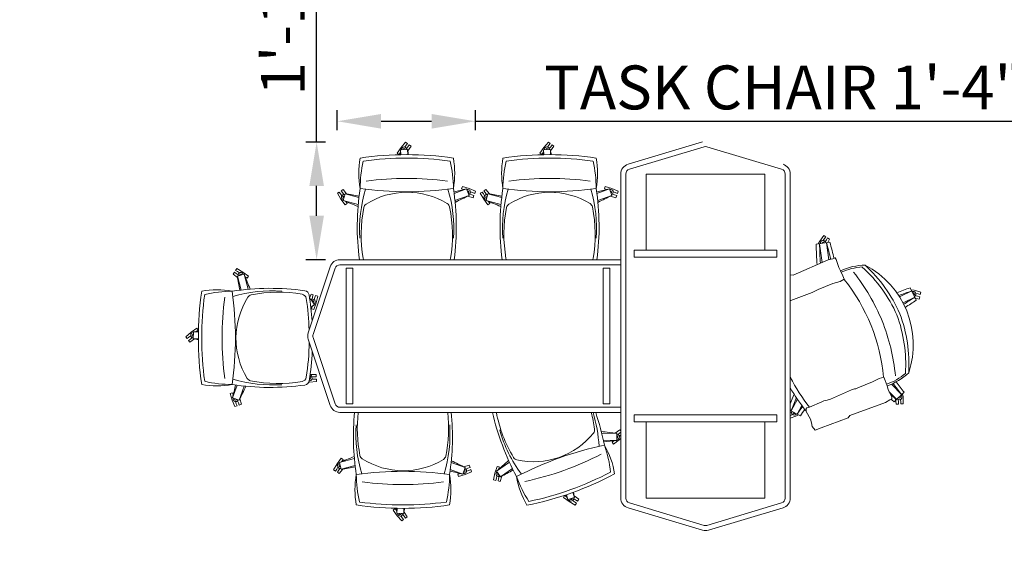
# Model space of a CAD drawing. Units: inches. Extents: x -100 to 766, y -562 to 63.
# Tile 5 of 11: x 268 to 380, y -383 to -323. Entities that reach past the tile are written whole.
import ezdxf

# ---------------------------------------------------------------- set-up
doc = ezdxf.new("R2010")
doc.units = ezdxf.units.IN
doc.layers.add('A-ANNO-DIMS', color=2, linetype='Continuous', lineweight=18)
doc.layers.add('furn', color=8, linetype='Continuous', lineweight=13)
doc.styles.get("Standard").update_dxf_attribs({"font": 'arial.ttf'})
doc.dimstyles.new('ISO-25', dxfattribs={"dimtxt": 5, "dimasz": 5, "dimexe": 1.25, "dimexo": 0.625, "dimtad": 1, "dimlunit": 3, "dimtxsty": 'Standard', "dimcen": 2.5, "dimadec": 0, "dimazin": 0, "dimtfac": 1, "dimtmove": 0, "dimatfit": 3, "dimfxl": 1, "dimfxlon": 1, "dimarcsym": 0})

# ---------------------------------------------------------------- blocks, each defined once
blk = doc.blocks.new('CHAIR-OFFICE')
for p, q in [((6.82, 12.16), (7.28, 12.81)), ((7.22, 12.53), (8.02, 12.56)), ((7.22, 12.53), (7.25, 11.97)), ((7.28, 12.81), (7.79, 13.42)), ((7.84, 13.05), (7.68, 12.84)), ((7.79, 13.42), (8, 13.25)), ((8, 13.25), (7.84, 13.05)), ((8.05, 12.88), (7.89, 12.68)), ((8.02, 12.56), (8.04, 11.98)), ((8.04, 12.4), (8.42, 12.93)), ((8.21, 13.09), (8.05, 12.88)), ((8.42, 12.93), (8.21, 13.09)), ((7.03, 12), (6.82, 12.16)), ((7.19, 12.21), (7.03, 12)), ((7.2, 12.22), (7.19, 12.21)), ((0.66, 8.02), (0.44, 7.87)), ((0.44, 7.87), (0.59, 7.65)), ((1.05, 7.5), (0.66, 8.02)), ((14.74, 8.08), (13.32, 7.55)), ((14.18, 8.1), (14.27, 8.35)), ((14.43, 8.01), (14.18, 8.1)), ((14.27, 8.35), (15.03, 8.12)), ((14.43, 8.01), (14.43, 8.01)), ((14.74, 8.08), (15.02, 7.34)), ((15.03, 8.12), (15.76, 7.81)), ((0, 7.57), (0.22, 7.72)), ((0.41, 6.89), (0, 7.57)), ((0.22, 7.72), (0.37, 7.5)), ((0.37, 7.5), (0.51, 7.29)), ((0.89, 6.26), (0.41, 6.89)), ((0.59, 7.65), (0.73, 7.44)), ((0.67, 6.76), (0.88, 7.52)), ((0.67, 6.76), (2.38, 6.28)), ((0.88, 7.52), (2.46, 7.08)), ((15.02, 7.34), (13.41, 6.74)), ((14.87, 7.26), (15.49, 7.07)), ((15.33, 7.4), (15.09, 7.49)), ((15.42, 7.65), (15.18, 7.74)), ((15.58, 7.32), (15.33, 7.4)), ((15.67, 7.56), (15.42, 7.65)), ((15.49, 7.07), (15.58, 7.32)), ((15.76, 7.81), (15.67, 7.56)), ((1.11, 6.41), (0.89, 6.26)), ((0.96, 6.64), (0.96, 6.63)), ((0.96, 6.63), (1.11, 6.41))]:
    blk.add_line(p, q)
for centre, radius, start, end in [((54.31, 8.3), 47.27, 174.8588, 175.5421), ((7.62, 12.55), 0.303, 2.3066, 182.3066), ((7.62, 12.55), 0.132, 2.3066, 182.3066), ((-38.57, 4.55), 47.27, 9.0337, 9.7544), ((25.26, -38.01), 47.27, 102.8588, 104.6675), ((14.88, 7.71), 0.303, 290.3066, 110.3066), ((0.77, 7.14), 0.303, 74.3066, 254.3066), ((0.77, 7.14), 0.132, 74.3066, 254.3066), ((19.24, 50.23), 47.27, 246.8588, 249.0775), ((-5.9, -39.26), 47.27, 79.7853, 81.7544), ((-7, 49.17), 47.27, 295.6055, 297.7544), ((14.88, 7.71), 0.132, 290.3066, 110.3066)]:
    blk.add_arc(centre, radius, start, end)
at = {"ltscale": 0.7}
for centre, radius, start, end in [((12.2, 9.85), 9.75, 169.7192, 190.2808), ((7.92, -24.77), 36.75, 81.6807, 98.3193), ((16.39, 8.11), 13.79, 166.8278, 180), ((7.92, -24.77), 36.36, 82.1689, 97.8311), ((-0.55, 8.11), 13.79, 0, 13.1722), ((3.64, 9.85), 9.75, 349.7192, 10.2808), ((7.92, -24.77), 34.04, 82.1689, 97.8311), ((30.98, 3.76), 28.71, 171.2841, 187.5243), ((18.22, 3.49), 15.68, 163.1781, 183.7805), ((7.92, 47.15), 39.4, 262.2438, 277.7562), ((-2.39, 3.49), 15.68, 356.2195, 16.8219), ((-15.14, 3.76), 28.71, 352.4757, 8.7159), ((7.96, -1.07), 8.76, 58.484, 122.3392), ((18.36, 2.85), 15.65, 168.5812, 189.9952), ((3.59, 5.84), 0.58, 122.3392, 168.5812), ((12.24, 5.9), 0.58, 11.6599, 58.484), ((-2.52, 2.85), 15.65, 350.0048, 11.6599), ((3.52, 0.24), 0.58, 189.9952, 204.0918), ((12.32, 0.24), 0.58, 335.9082, 350.0048)]:
    blk.add_arc(centre, radius, start, end, dxfattribs=at)
blk = doc.blocks.new('*D32')
at = {"layer": 'A-ANNO-DIMS', "color": 0, "lineweight": -2, "transparency": 16777216}
for p, q in [((304.17, -335.87), (304.17, -333.62)), ((319.93, -335.87), (319.93, -333.62)), ((309.17, -334.87), (314.93, -334.87)), ((319.93, -334.87), (400.64, -334.87))]:
    blk.add_line(p, q, dxfattribs=at)
at = {"layer": 'A-ANNO-DIMS', "color": 0, "transparency": 16777216}
for points in [[(309.17, -334.04), (309.17, -335.71), (304.17, -334.87)], [(314.93, -334.04), (314.93, -335.71), (319.93, -334.87)]]:
    blk.add_solid(points, dxfattribs=at)
at = {"layer": 'Defpoints', "color": 0, "transparency": 16777216}
for p in [(319.93, -334.87), (304.17, -337.24), (319.93, -337.24)]:
    blk.add_point(p, dxfattribs=at)
at = {"layer": 'A-ANNO-DIMS', "color": 0, "transparency": 16777216, "insert": (362.79, -331.66), "char_height": 5, "attachment_point": 5}
blk.add_mtext('TASK CHAIR 1\'-4" TYP.', dxfattribs=at)
blk = doc.blocks.new('*D33')
at = {"layer": 'A-ANNO-DIMS', "color": 0, "lineweight": -2, "transparency": 16777216}
for p, q in [((301.81, -337.24), (301.81, -289.33)), ((302.81, -337.24), (300.56, -337.24)), ((301.81, -345.65), (301.81, -342.24)), ((302.81, -350.65), (300.56, -350.65))]:
    blk.add_line(p, q, dxfattribs=at)
at = {"layer": 'A-ANNO-DIMS', "color": 0, "transparency": 16777216}
for points in [[(300.98, -342.24), (302.64, -342.24), (301.81, -337.24)], [(300.98, -345.65), (302.64, -345.65), (301.81, -350.65)]]:
    blk.add_solid(points, dxfattribs=at)
at = {"layer": 'Defpoints', "color": 0, "transparency": 16777216}
for p in [(301.81, -337.24), (304.17, -337.24), (304.17, -350.65)]:
    blk.add_point(p, dxfattribs=at)
at = {"layer": 'A-ANNO-DIMS', "color": 0, "transparency": 16777216, "insert": (298.6, -310.78), "char_height": 5, "attachment_point": 5, "rotation": 90}
blk.add_mtext('1\'-1 1/2" TYP.', dxfattribs=at)
blk = doc.blocks.new('*D49')
at = {"layer": 'A-ANNO-DIMS', "color": 0, "lineweight": -2, "transparency": 16777216}
for p, q in [((-88.51, -356.21), (-90.76, -356.21)), ((-89.51, -361.21), (-89.51, -417.21)), ((-88.51, -422.21), (-90.76, -422.21))]:
    blk.add_line(p, q, dxfattribs=at)
at = {"layer": 'A-ANNO-DIMS', "color": 0, "transparency": 16777216}
for points in [[(-90.35, -361.21), (-88.68, -361.21), (-89.51, -356.21)], [(-90.35, -417.21), (-88.68, -417.21), (-89.51, -422.21)]]:
    blk.add_solid(points, dxfattribs=at)
at = {"layer": 'Defpoints', "color": 0, "transparency": 16777216}
for p in [(562.39, -356.21), (-89.51, -422.21), (562.39, -422.21)]:
    blk.add_point(p, dxfattribs=at)
at = {"layer": 'A-ANNO-DIMS', "color": 0, "transparency": 16777216, "insert": (-92.69, -389.21), "char_height": 5, "attachment_point": 5, "rotation": 90}
blk.add_mtext('5\'-6"', dxfattribs=at)
blk = doc.blocks.new('*D51')
at = {"layer": 'A-ANNO-DIMS', "color": 0, "lineweight": -2, "transparency": 16777216}
for p, q in [((-88.51, -308.21), (-90.76, -308.21)), ((-89.51, -313.21), (-89.51, -339.21)), ((-88.51, -344.21), (-90.76, -344.21))]:
    blk.add_line(p, q, dxfattribs=at)
at = {"layer": 'A-ANNO-DIMS', "color": 0, "transparency": 16777216}
for points in [[(-90.35, -313.21), (-88.68, -313.21), (-89.51, -308.21)], [(-90.35, -339.21), (-88.68, -339.21), (-89.51, -344.21)]]:
    blk.add_solid(points, dxfattribs=at)
at = {"layer": 'Defpoints', "color": 0, "transparency": 16777216}
for p in [(598.6, -308.21), (-89.51, -344.21), (598.6, -344.21)]:
    blk.add_point(p, dxfattribs=at)
at = {"layer": 'A-ANNO-DIMS', "color": 0, "transparency": 16777216, "insert": (-92.69, -326.21), "char_height": 5, "attachment_point": 5, "rotation": 90}
blk.add_mtext('3\'-0"', dxfattribs=at)
blk = doc.blocks.new('*D70')
at = {"layer": 'A-ANNO-DIMS', "color": 0, "lineweight": -2, "transparency": 16777216}
for p, q in [((-88.51, -376.85), (-90.76, -376.85)), ((-89.51, -381.85), (-89.51, -419.34)), ((-88.51, -424.34), (-90.76, -424.34))]:
    blk.add_line(p, q, dxfattribs=at)
at = {"layer": 'A-ANNO-DIMS', "color": 0, "transparency": 16777216}
for points in [[(-90.35, -381.85), (-88.68, -381.85), (-89.51, -376.85)], [(-90.35, -419.34), (-88.68, -419.34), (-89.51, -424.34)]]:
    blk.add_solid(points, dxfattribs=at)
at = {"layer": 'Defpoints', "color": 0, "transparency": 16777216}
for p in [(679.5, -376.85), (-89.51, -424.34), (679.5, -424.34)]:
    blk.add_point(p, dxfattribs=at)
at = {"layer": 'A-ANNO-DIMS', "color": 0, "transparency": 16777216, "insert": (-92.73, -400.59), "char_height": 5, "attachment_point": 5, "rotation": 90}
blk.add_mtext('3\'-11 1/2"', dxfattribs=at)
blk = doc.blocks.new('*D73')
at = {"layer": 'A-ANNO-DIMS', "color": 0, "lineweight": -2, "transparency": 16777216}
for p, q in [((-88.51, -345.04), (-90.76, -345.04)), ((-89.51, -350.04), (-89.51, -401.82)), ((-88.51, -406.82), (-90.76, -406.82))]:
    blk.add_line(p, q, dxfattribs=at)
at = {"layer": 'A-ANNO-DIMS', "color": 0, "transparency": 16777216}
for points in [[(-90.35, -350.04), (-88.68, -350.04), (-89.51, -345.04)], [(-90.35, -401.82), (-88.68, -401.82), (-89.51, -406.82)]]:
    blk.add_solid(points, dxfattribs=at)
at = {"layer": 'Defpoints', "color": 0, "transparency": 16777216}
for p in [(475.3, -345.04), (-89.51, -406.82), (475.3, -406.82)]:
    blk.add_point(p, dxfattribs=at)
at = {"layer": 'A-ANNO-DIMS', "color": 0, "transparency": 16777216, "insert": (-92.69, -375.93), "char_height": 5, "attachment_point": 5, "rotation": 90}
blk.add_mtext('5\'-2"', dxfattribs=at)
blk = doc.blocks.new('*D80')
at = {"layer": 'A-ANNO-DIMS', "color": 0, "lineweight": -2, "transparency": 16777216}
for p, q in [((241.52, -558.16), (236.52, -558.16)), ((246.52, -557.16), (246.52, -559.41)), ((246.52, -558.16), (250.39, -558.16)), ((250.39, -557.16), (250.39, -559.41)), ((255.39, -558.16), (274.93, -558.16))]:
    blk.add_line(p, q, dxfattribs=at)
at = {"layer": 'A-ANNO-DIMS', "color": 0, "transparency": 16777216}
for points in [[(241.52, -557.32), (241.52, -558.99), (246.52, -558.16)], [(255.39, -557.32), (255.39, -558.99), (250.39, -558.16)]]:
    blk.add_solid(points, dxfattribs=at)
at = {"layer": 'Defpoints', "color": 0, "transparency": 16777216}
for p in [(246.52, -368.21), (250.39, -368.21), (250.39, -558.16)]:
    blk.add_point(p, dxfattribs=at)
at = {"layer": 'A-ANNO-DIMS', "color": 0, "transparency": 16777216, "insert": (267.66, -554.98), "char_height": 5, "attachment_point": 5}
blk.add_mtext('0\'-4"', dxfattribs=at)
blk = doc.blocks.new('*D87')
at = {"layer": 'A-ANNO-DIMS', "color": 0, "lineweight": -2, "transparency": 16777216}
for p, q in [((310.41, -557.16), (310.41, -559.41)), ((315.41, -558.16), (352.79, -558.16)), ((357.79, -557.16), (357.79, -559.41))]:
    blk.add_line(p, q, dxfattribs=at)
at = {"layer": 'A-ANNO-DIMS', "color": 0, "transparency": 16777216}
for points in [[(315.41, -557.32), (315.41, -558.99), (310.41, -558.16)], [(352.79, -557.32), (352.79, -558.99), (357.79, -558.16)]]:
    blk.add_solid(points, dxfattribs=at)
at = {"layer": 'Defpoints', "color": 0, "transparency": 16777216}
for p in [(310.41, -121.91), (357.79, -121.91), (357.79, -558.16)]:
    blk.add_point(p, dxfattribs=at)
at = {"layer": 'A-ANNO-DIMS', "color": 0, "transparency": 16777216, "insert": (334.1, -554.94), "char_height": 5, "attachment_point": 5}
blk.add_mtext('3\'-11 1/2"', dxfattribs=at)

msp = doc.modelspace()

# ---------------------------------------------------------------- linework, layer by layer
at = {"layer": 'furn', "ltscale": 0.2}
for p, q in [((337.331, -339.771), (345.839, -337.219)), ((337.498, -340.326), (346.006, -337.774)), ((346.339, -337.774), (354.847, -340.326)), ((336.504, -377.828), (336.504, -340.882)), ((337.084, -377.828), (337.084, -340.882)), ((355.26, -340.882), (355.26, -377.828)), ((355.84, -340.882), (355.84, -377.828)), ((300.855, -358.988), (303.369, -351.447)), ((304.469, -350.654), (336.504, -350.654)), ((304.469, -351.234), (336.504, -351.234)), ((336.504, -350.654), (336.504, -368.056)), ((301.405, -359.171), (303.919, -351.63)), ((303.369, -367.263), (300.855, -359.722)), ((303.919, -367.079), (301.405, -359.538)), ((336.504, -367.476), (304.469, -367.476)), ((336.504, -368.056), (304.469, -368.056)), ((346.006, -380.935), (337.498, -378.383)), ((354.847, -378.383), (346.339, -380.935)), ((345.839, -381.491), (337.331, -378.939)), ((355.013, -378.939), (346.506, -381.491))]:
    msp.add_line(p, q, dxfattribs=at)
at = {"layer": 'furn', "ltscale": 0.4}
for p, q in [((339.405, -349.583), (339.405, -340.882)), ((339.405, -340.882), (349.073, -340.882)), ((349.073, -340.882), (352.94, -340.882)), ((352.94, -340.882), (352.94, -349.583)), ((338.051, -349.583), (354.293, -349.583)), ((338.051, -350.357), (338.051, -349.583)), ((354.293, -350.357), (338.051, -350.357)), ((352.94, -349.583), (339.405, -349.583)), ((354.293, -349.583), (354.293, -350.357)), ((305.944, -351.62), (305.171, -351.62)), ((305.171, -351.62), (305.171, -367.089)), ((305.944, -367.089), (305.944, -351.62)), ((335.259, -351.62), (334.486, -351.62)), ((334.486, -351.62), (334.486, -367.089)), ((335.259, -367.089), (335.259, -351.62)), ((305.171, -367.089), (305.944, -367.089)), ((334.486, -367.089), (335.259, -367.089)), ((354.293, -368.353), (338.051, -368.353)), ((338.051, -368.353), (338.051, -369.126)), ((354.293, -369.126), (354.293, -368.353)), ((338.051, -369.126), (354.293, -369.126)), ((339.405, -369.126), (339.405, -377.828)), ((352.94, -369.126), (339.405, -369.126)), ((352.94, -377.828), (352.94, -369.126)), ((339.405, -377.828), (349.073, -377.828)), ((349.073, -377.828), (352.94, -377.828))]:
    msp.add_line(p, q, dxfattribs=at)
at = {"layer": 'furn'}
for p, q in [((359.208, -348.542), (359.659, -347.889)), ((359.659, -347.889), (359.883, -348.028)), ((359.883, -348.028), (359.744, -348.253)), ((360.107, -348.167), (359.968, -348.392)), ((360.332, -348.306), (360.107, -348.167)), ((358.801, -348.885), (360.356, -348.657)), ((359.038, -348.85), (359.208, -348.542)), ((359.187, -348.829), (359.5, -350.966)), ((359.193, -349.143), (359.188, -349.15)), ((359.744, -348.253), (359.61, -348.469)), ((359.968, -348.392), (359.834, -348.608)), ((359.97, -348.714), (360.256, -350.66)), ((360.119, -348.692), (360.332, -348.306)), ((292.275, -352.3), (292.424, -352.082)), ((292.796, -352.694), (292.275, -352.3)), ((292.424, -352.082), (292.642, -352.23)), ((292.72, -351.645), (292.572, -351.864)), ((292.572, -351.864), (292.79, -352.012)), ((292.642, -352.23), (292.853, -352.374)), ((293.397, -352.058), (292.72, -351.645)), ((293.534, -352.311), (292.772, -352.525)), ((292.772, -352.525), (293.216, -354.107)), ((292.79, -352.012), (293.001, -352.155)), ((294.03, -352.535), (293.397, -352.058)), ((293.534, -352.311), (294.016, -354.025)), ((293.657, -352.601), (293.664, -352.605)), ((293.664, -352.605), (293.882, -352.754)), ((293.882, -352.754), (294.03, -352.535)), ((301.015, -355.043), (301.176, -354.575)), ((301.176, -354.575), (301.43, -354.649)), ((301.356, -354.902), (301.285, -355.147)), ((301.43, -354.649), (301.356, -354.902)), ((301.683, -354.722), (301.61, -354.976)), ((301.937, -354.796), (301.683, -354.722)), ((301.754, -355.567), (301.937, -354.796)), ((369.696, -354.207), (368.312, -354.893)), ((370.048, -354.917), (368.707, -355.581)), ((369.399, -354.31), (369.391, -354.308)), ((369.523, -353.858), (370.221, -355.266)), ((369.629, -354.072), (369.976, -354.139)), ((369.976, -354.139), (370.735, -354.366)), ((370.353, -354.816), (370.106, -354.755)), ((370.416, -354.559), (370.169, -354.499)), ((370.61, -354.878), (370.353, -354.816)), ((370.672, -354.622), (370.416, -354.559)), ((370.547, -355.135), (370.61, -354.878)), ((370.735, -354.366), (370.672, -354.622)), ((301.116, -355.116), (301.034, -355.171)), ((301.555, -355.775), (301.116, -355.116)), ((301.555, -355.775), (301.15, -356.046)), ((301.315, -355.99), (301.242, -356.243)), ((301.317, -355.982), (301.315, -355.99)), ((301.495, -356.317), (301.754, -355.567)), ((301.61, -354.976), (301.539, -355.22)), ((369.906, -355.011), (370.547, -355.135)), ((301.242, -356.243), (301.495, -356.317)), ((287.478, -358.921), (286.876, -359.437)), ((286.876, -359.437), (287.038, -359.646)), ((287.246, -359.484), (287.448, -359.328)), ((288.127, -358.466), (287.478, -358.921)), ((287.76, -358.869), (287.728, -359.66)), ((287.76, -358.869), (288.321, -358.892)), ((288.074, -358.842), (288.081, -358.837)), ((288.081, -358.837), (288.289, -358.675)), ((288.289, -358.675), (288.127, -358.466)), ((287.038, -359.646), (287.246, -359.484)), ((287.2, -359.854), (287.408, -359.692)), ((287.361, -360.063), (287.2, -359.854)), ((287.896, -359.689), (287.361, -360.063)), ((287.408, -359.692), (287.609, -359.536)), ((287.728, -359.66), (288.315, -359.684)), ((301.007, -364.136), (301.23, -363.853)), ((301.007, -364.136), (301.23, -363.853)), ((301.23, -363.853), (301.067, -363.725)), ((301.23, -363.853), (301.067, -363.725)), ((301.111, -363.731), (301.763, -363.743)), ((301.111, -363.731), (301.763, -363.743)), ((301.763, -363.743), (301.772, -364.007)), ((301.763, -363.743), (301.772, -364.007)), ((292.213, -366.387), (292.741, -364.961)), ((300.915, -364.598), (300.998, -364.599)), ((300.915, -364.598), (300.998, -364.599)), ((300.998, -364.599), (301.788, -364.535)), ((300.998, -364.599), (301.788, -364.535)), ((301.508, -364.015), (301.253, -364.023)), ((301.508, -364.015), (301.253, -364.023)), ((301.516, -364.279), (301.262, -364.287)), ((301.516, -364.279), (301.262, -364.287)), ((301.772, -364.007), (301.508, -364.015)), ((301.772, -364.007), (301.508, -364.015)), ((301.78, -364.271), (301.516, -364.279)), ((301.78, -364.271), (301.516, -364.279)), ((301.788, -364.535), (301.78, -364.271)), ((301.788, -364.535), (301.78, -364.271)), ((368.554, -366.044), (367.379, -364.841)), ((292.192, -365.824), (291.944, -365.913)), ((291.944, -365.913), (292.175, -366.671)), ((292.282, -366.072), (292.192, -365.824)), ((292.284, -366.08), (292.282, -366.072)), ((292.956, -366.661), (293.55, -365.057)), ((367.988, -366.597), (367.141, -365.731)), ((368.833, -365.771), (367.709, -366.87)), ((368.364, -365.792), (368.363, -365.784)), ((368.661, -365.938), (368.705, -366.288)), ((292.175, -366.671), (292.48, -367.403)), ((292.213, -366.387), (292.956, -366.661)), ((292.639, -367.065), (292.553, -366.826)), ((292.729, -367.314), (292.639, -367.065)), ((292.888, -366.976), (292.801, -366.736)), ((292.977, -367.224), (292.888, -366.976)), ((293.225, -367.135), (292.977, -367.224)), ((293.035, -366.51), (293.225, -367.135)), ((355.945, -367.894), (356.653, -366.543)), ((356.646, -368.262), (357.166, -367.27)), ((367.854, -366.491), (367.934, -367.139)), ((367.934, -367.139), (368.198, -367.12)), ((368.178, -366.857), (368.159, -366.602)), ((368.198, -367.12), (368.178, -366.857)), ((368.441, -366.837), (368.423, -366.583)), ((368.461, -367.1), (368.441, -366.837)), ((368.724, -367.081), (368.461, -367.1)), ((368.705, -366.288), (368.724, -367.081)), ((292.48, -367.403), (292.729, -367.314)), ((356.004, -367.734), (355.84, -367.811)), ((356.992, -368.443), (355.84, -367.84)), ((355.84, -368.122), (355.993, -368.059)), ((355.84, -368.407), (355.857, -368.4)), ((355.857, -368.4), (356.093, -368.304)), ((356.779, -368.332), (356.46, -368.481)), ((356.826, -368.004), (356.834, -368)), ((356.46, -368.481), (355.84, -368.699)), ((336.048, -370.46), (334.337, -370.442)), ((335.879, -370.437), (336.403, -370.047)), ((336.04, -371.252), (336.048, -370.46)), ((336.367, -370.418), (336.17, -370.58)), ((336.504, -370.647), (336.338, -370.784)), ((336.504, -370.305), (336.367, -370.418)), ((336.403, -370.047), (336.504, -370.17)), ((336.04, -371.252), (334.519, -371.236)), ((335.72, -371.294), (335.517, -371.462)), ((335.517, -371.462), (335.685, -371.665)), ((335.685, -371.665), (336.321, -371.192)), ((335.727, -371.288), (335.72, -371.294)), ((336.321, -371.192), (336.504, -371.024)), ((304.149, -373.918), (303.737, -374.595)), ((304.627, -373.285), (304.149, -373.918)), ((304.402, -373.781), (306.116, -373.3)), ((304.402, -373.781), (304.616, -374.543)), ((304.845, -373.433), (304.627, -373.285)), ((304.692, -373.658), (304.697, -373.651)), ((304.697, -373.651), (304.845, -373.433)), ((318.753, -374.359), (317.148, -373.765)), ((322.343, -374.756), (323.794, -373.725)), ((303.737, -374.595), (303.955, -374.743)), ((303.955, -374.743), (304.104, -374.525)), ((304.104, -374.525), (304.247, -374.314)), ((304.174, -374.891), (304.322, -374.673)), ((304.392, -375.04), (304.174, -374.891)), ((304.322, -374.673), (304.465, -374.462)), ((304.785, -374.519), (304.392, -375.04)), ((304.616, -374.543), (306.198, -374.099)), ((318.478, -375.102), (317.052, -374.574)), ((318.164, -375.033), (317.915, -375.123)), ((317.915, -375.123), (318.005, -375.371)), ((318.005, -375.371), (318.763, -375.14)), ((318.171, -375.031), (318.164, -375.033)), ((318.478, -375.102), (318.753, -374.359)), ((318.602, -374.28), (319.226, -374.09)), ((318.763, -375.14), (319.495, -374.835)), ((319.067, -374.427), (318.828, -374.514)), ((319.157, -374.676), (318.917, -374.762)), ((319.316, -374.338), (319.067, -374.427)), ((319.405, -374.586), (319.157, -374.676)), ((319.226, -374.09), (319.316, -374.338)), ((319.495, -374.835), (319.405, -374.586)), ((322.151, -374.97), (321.991, -375.747)), ((322.387, -374.213), (322.151, -374.97)), ((322.343, -374.756), (322.802, -375.402)), ((322.643, -374.279), (322.387, -374.213)), ((322.575, -374.543), (322.577, -374.535)), ((322.577, -374.535), (322.643, -374.279)), ((322.802, -375.402), (324.141, -374.45)), ((321.991, -375.747), (322.247, -375.813)), ((322.247, -375.813), (322.313, -375.557)), ((322.313, -375.557), (322.377, -375.311)), ((322.502, -375.879), (322.568, -375.623)), ((322.758, -375.945), (322.502, -375.879)), ((322.568, -375.623), (322.632, -375.377)), ((322.952, -375.322), (322.758, -375.945)), ((331.22, -377.743), (331.045, -377.183)), ((330.103, -377.547), (329.962, -377.77)), ((329.962, -377.77), (330.609, -378.228)), ((330.326, -377.689), (330.103, -377.547)), ((330.465, -377.98), (330.297, -377.444)), ((330.333, -377.694), (330.326, -377.689)), ((330.465, -377.98), (331.22, -377.743)), ((330.609, -378.228), (331.298, -378.62)), ((331.217, -378.256), (331.002, -378.119)), ((331.358, -378.033), (331.144, -377.897)), ((331.19, -377.575), (331.723, -377.952)), ((331.439, -378.398), (331.217, -378.256)), ((331.298, -378.62), (331.439, -378.398)), ((331.581, -378.175), (331.358, -378.033)), ((331.723, -377.952), (331.581, -378.175)), ((310.766, -379.026), (310.558, -379.188)), ((310.558, -379.188), (311.012, -379.838)), ((310.928, -379.235), (310.766, -379.026)), ((310.933, -379.241), (310.928, -379.235)), ((310.96, -379.555), (310.983, -378.994)), ((310.96, -379.555), (311.752, -379.587)), ((311.752, -379.587), (311.775, -379)), ((311.78, -379.419), (312.154, -379.954)), ((311.012, -379.838), (311.529, -380.439)), ((311.575, -380.069), (311.419, -379.867)), ((311.529, -380.439), (311.737, -380.277)), ((311.737, -380.277), (311.575, -380.069)), ((311.784, -379.907), (311.628, -379.706)), ((311.946, -380.115), (311.784, -379.907)), ((312.154, -379.954), (311.946, -380.115))]:
    msp.add_line(p, q, dxfattribs=at)
at = {"layer": 'furn', "ltscale": 0.7}
for p, q in [((356.171, -352.424), (360.148, -350.682)), ((360.148, -350.682), (360.701, -350.565)), ((360.701, -350.565), (360.95, -350.453)), ((360.95, -350.453), (361.085, -350.61)), ((361.085, -350.61), (361.382, -351.551)), ((361.382, -351.551), (361.584, -351.905)), ((355.84, -352.391), (355.882, -352.373)), ((355.882, -352.373), (356.171, -352.424)), ((361.584, -351.905), (361.836, -352.499)), ((361.836, -352.499), (361.988, -352.874)), ((360.708, -353.379), (359.006, -354.067)), ((361.522, -353.121), (360.708, -353.379)), ((361.988, -352.874), (361.522, -353.121)), ((358.358, -354.388), (355.891, -355.305)), ((358.654, -354.245), (358.358, -354.388)), ((358.804, -354.149), (358.654, -354.245)), ((359.006, -354.067), (358.804, -354.149)), ((355.891, -355.305), (355.84, -355.333)), ((365.237, -364.586), (363.535, -365.273)), ((366.002, -364.206), (365.237, -364.586)), ((366.508, -364.06), (366.002, -364.206)), ((366.66, -364.435), (366.508, -364.06)), ((366.891, -365.037), (366.66, -364.435)), ((366.992, -365.432), (366.891, -365.037)), ((362.846, -365.493), (360.435, -366.547)), ((363.158, -365.39), (362.846, -365.493)), ((363.333, -365.355), (363.158, -365.39)), ((363.535, -365.273), (363.333, -365.355)), ((367.432, -366.315), (366.992, -365.432)), ((359.451, -366.852), (358.054, -367.48)), ((359.681, -366.736), (359.451, -366.852)), ((360.062, -366.652), (359.681, -366.736)), ((360.435, -366.547), (360.062, -366.652)), ((362.638, -368.425), (366.708, -366.914)), ((366.708, -366.914), (367.187, -366.614)), ((367.187, -366.614), (367.445, -366.522)), ((367.445, -366.522), (367.432, -366.315)), ((357.739, -367.54), (357.642, -367.602)), ((357.642, -367.602), (357.655, -367.957)), ((357.655, -367.957), (358.134, -368.837)), ((357.894, -367.505), (357.739, -367.54)), ((358.054, -367.48), (357.894, -367.505)), ((358.134, -368.837), (358.276, -369.231)), ((358.276, -369.231), (358.35, -369.677)), ((359.368, -369.824), (362.465, -368.662)), ((362.465, -368.662), (362.638, -368.425)), ((358.35, -369.677), (358.685, -370.1)), ((358.685, -370.1), (359.368, -369.824))]:
    msp.add_line(p, q, dxfattribs=at)
at = {"layer": 'furn', "ltscale": 0.2}
for centre, radius, start, end in [((346.172, -338.33), 0.58, 73.30076, 106.69924), ((337.664, -340.882), 1.16, 106.69924, 180), ((337.664, -340.882), 0.58, 106.69924, 180), ((354.68, -340.882), 0.58, 0, 73.30076), ((354.68, -340.882), 1.16, 0, 73.30076), ((304.469, -351.814), 1.16, 90, 161.56505), ((304.469, -351.814), 0.58, 90, 161.56505), ((301.956, -359.355), 1.16, 161.56505, 198.43495), ((301.956, -359.355), 0.58, 161.56505, 198.43495), ((304.469, -366.896), 1.16, 198.43495, 270), ((304.469, -366.896), 0.58, 198.43495, 270), ((337.664, -377.828), 1.16, 180, 253.30076), ((337.664, -377.828), 0.58, 180, 253.30076), ((354.68, -377.828), 0.58, 286.69924, 0), ((354.68, -377.828), 1.16, 286.69924, 0), ((346.172, -380.38), 1.16, 253.30076, 286.69924), ((346.172, -380.38), 0.58, 253.30076, 286.69924)]:
    msp.add_arc(centre, radius, start, end, dxfattribs=at)
at = {"layer": 'furn'}
for centre, radius, start, end in [((406.454, -348.084), 47.66, 180.963, 183.7842), ((406.454, -348.084), 47.273, 180.90223, 183.61481), ((359.578, -348.771), 0.303, 8.35, 188.35), ((359.578, -348.771), 0.132, 8.35, 188.35), ((314.482, -361.583), 47.273, 13.41608, 15.79778), ((314.482, -361.583), 47.66, 13.41608, 15.73701), ((339.556, -345.745), 47.273, 188.2456, 190.21466), ((293.153, -352.418), 0.303, 15.69338, 195.69338), ((293.153, -352.418), 0.132, 15.69338, 195.69338), ((250.064, -370.889), 47.273, 20.92253, 23.14116), ((385.011, -398.931), 47.66, 108.963, 110.92121), ((385.011, -398.931), 47.273, 108.90223, 110.81068), ((343.751, -315.632), 47.273, 301.97499, 303.79778), ((369.872, -354.562), 0.303, 296.35, 116.35), ((369.872, -354.562), 0.132, 296.35, 116.35), ((322.021, -397.516), 47.273, 116.2456, 116.35919), ((270.453, -320.174), 47.273, 310.5051, 311.14116), ((301.336, -355.446), 0.303, 303.69338, 123.69338), ((301.336, -355.446), 0.132, 303.69338, 123.69338), ((343.751, -315.632), 47.66, 301.92298, 303.73701), ((287.744, -359.265), 0.303, 87.69338, 267.69338), ((287.744, -359.265), 0.132, 87.69338, 267.69338), ((291.996, -405.952), 47.273, 94.45788, 95.14116), ((295.738, -313.07), 47.273, 260.2456, 260.96632), ((300.984, -364.164), 0.303, 264.2846, 51.69338), ((300.984, -364.164), 0.303, 264.2846, 51.69338), ((267.365, -396.837), 47.273, 44.2456, 44.51988), ((267.365, -396.837), 47.273, 44.2456, 44.51988), ((338.301, -376.907), 47.273, 165.33246, 167.14116), ((300.984, -364.164), 0.132, 268.83313, 51.69338), ((300.984, -364.164), 0.132, 268.83313, 51.69338), ((330.751, -394.429), 47.273, 36.90223, 38.87325), ((330.751, -394.429), 47.66, 36.963, 38.7754), ((251.121, -344.647), 47.273, 332.2456, 334.39454), ((400.31, -384.219), 47.66, 157.49042, 158.91682), ((397.223, -329.448), 47.273, 230.72258, 231.79778), ((368.271, -366.32), 0.303, 224.35, 44.35), ((292.585, -366.524), 0.303, 159.69338, 339.69338), ((292.585, -366.524), 0.132, 159.69338, 339.69338), ((400.31, -384.219), 47.273, 157.81448, 159.79778), ((397.223, -329.448), 47.66, 231.14855, 231.73701), ((368.271, -366.32), 0.132, 224.35, 44.35), ((356.295, -368.078), 0.303, 152.35, 332.35), ((356.295, -368.078), 0.132, 152.35, 332.35), ((317.969, -341.081), 47.273, 324.90223, 326.19386), ((317.969, -341.081), 47.66, 324.963, 326.03412), ((329.435, -417.268), 47.273, 81.95831, 84.10725), ((336.044, -370.856), 0.303, 269.40608, 89.40608), ((330.398, -324.316), 47.273, 275.04516, 276.85386), ((336.044, -370.856), 0.132, 269.40608, 89.40608), ((304.509, -374.162), 0.303, 105.69338, 285.69338), ((304.509, -374.162), 0.132, 105.69338, 285.69338), ((322.981, -417.251), 47.273, 110.92253, 113.14116), ((296.739, -416.194), 47.273, 62.2456, 64.39454), ((354.495, -409.412), 47.273, 130.63523, 132.85386), ((297.837, -327.759), 47.273, 278.2456, 280.21466), ((328.999, -329.014), 47.273, 255.33246, 257.14116), ((318.615, -374.73), 0.303, 249.69338, 69.69338), ((318.615, -374.73), 0.132, 249.69338, 69.69338), ((322.573, -375.079), 0.303, 125.40608, 305.40608), ((322.573, -375.079), 0.132, 125.40608, 305.40608), ((300.639, -333.646), 47.273, 297.95831, 299.92736), ((284.659, -385.918), 47.273, 9.95831, 10.67903), ((373.359, -358.11), 47.273, 204.17059, 204.85386), ((330.842, -377.861), 0.303, 197.40608, 17.40608), ((330.842, -377.861), 0.132, 197.40608, 17.40608), ((358.043, -375.319), 47.273, 184.45788, 185.14116), ((311.356, -379.571), 0.303, 177.69338, 357.69338), ((311.356, -379.571), 0.132, 177.69338, 357.69338), ((265.162, -371.577), 47.273, 350.2456, 350.96632)]:
    msp.add_arc(centre, radius, start, end, dxfattribs=at)
at = {"layer": 'furn', "ltscale": 0.7}
for centre, radius, start, end in [((364.576, -358.552), 7.289, 91.40115, 114.23532), ((364.576, -358.552), 7.095, 94.08643, 114.23532), ((353.29, -363.438), 16.08, 23.80386, 48.00597), ((353.218, -363.476), 16.532, 23.78704, 47.55372), ((359.631, -360.333), 10.244, 341.74338, 62.26911), ((345.577, -366.013), 22.363, 22.00624, 38.583), ((345.577, -366.013), 21.01, 5.42949, 38.583), ((325.065, -359.563), 36.75, 171.68072, 188.31928), ((290.442, -363.84), 9.751, 79.71923, 100.28077), ((325.065, -359.563), 36.364, 172.16886, 187.83114), ((292.182, -368.031), 13.785, 90, 103.17216), ((325.065, -359.563), 34.043, 172.16886, 187.83114), ((296.532, -382.624), 28.71, 82.13296, 98.71594), ((253.142, -359.563), 39.4, 352.24381, 7.75619), ((296.797, -369.867), 15.676, 86.21948, 106.82194), ((301.365, -359.607), 8.759, 147.66079, 211.516), ((294.455, -355.232), 0.58, 101.41884, 147.66079), ((297.439, -370.006), 15.653, 80.00482, 101.41884), ((300.055, -355.162), 0.58, 8.67601, 80.00482), ((300.383, -354.759), 0.58, 9.35255, 82.13296), ((271.214, -359.563), 30.142, 3.6091, 9.35255), ((271.214, -359.563), 29.755, 1.69041, 8.67601), ((352.933, -362.561), 16.08, 356.2257, 20.42781), ((352.855, -362.584), 16.532, 356.67795, 20.44463), ((345.577, -366.013), 22.363, 5.42949, 22.00624), ((271.214, -359.563), 29.755, 351.32399, 359.06079), ((271.214, -359.563), 30.142, 350.64745, 357.06846), ((364.425, -358.178), 7.095, 289.77717, 309.92606), ((364.425, -358.178), 7.289, 289.77717, 312.61134), ((290.442, -355.286), 9.751, 259.71923, 280.28077), ((292.182, -351.095), 13.785, 256.82784, 270), ((296.532, -336.502), 28.71, 261.28406, 277.86704), ((296.797, -349.259), 15.676, 253.17806, 273.78052), ((294.393, -363.882), 0.58, 211.516, 258.34006), ((297.439, -349.12), 15.653, 258.34006, 279.99518), ((300.055, -363.964), 0.58, 279.99518, 351.32399), ((300.383, -364.367), 0.58, 277.86704, 350.64745), ((375.031, -354.131), 21.597, 207.30205, 218.17743), ((375.031, -354.131), 22.177, 210.07641, 218.17743), ((334.716, -370.783), 28.71, 174.55006, 188.71594), ((322.098, -369.876), 15.653, 173.32221, 191.41884), ((301.212, -369.876), 15.653, 348.34006, 6.67779), ((288.594, -370.783), 28.71, 351.28406, 5.44994), ((349.869, -361.709), 28.71, 192.77218, 208.42865), ((337.684, -365.112), 15.653, 190.84215, 211.13155), ((318.023, -372.157), 15.653, 8.05276, 15.18692), ((318.37, -372.714), 15.676, 2.89076, 17.28473), ((306.45, -377.266), 28.71, 10.99676, 18.7112), ((321.959, -370.518), 15.676, 176.21948, 196.82194), ((301.351, -370.518), 15.676, 343.17806, 3.78052), ((337.77, -365.762), 15.676, 195.93218, 216.53464), ((326.57, -364.924), 8.759, 257.37349, 321.2287), ((332.947, -370.045), 0.58, 321.2287, 8.05276), ((342.795, -410.335), 39.4, 101.95651, 117.4689), ((321.655, -376.439), 13.785, 6.54054, 19.7127), ((326.188, -376.664), 9.751, 9.43193, 29.99347), ((318.535, -342.627), 34.043, 281.88157, 297.54384), ((307.323, -372.86), 0.58, 191.41884, 237.66079), ((311.698, -365.95), 8.759, 237.66079, 301.516), ((315.974, -372.922), 0.58, 301.516, 348.34006), ((324.782, -372.904), 0.58, 211.13155, 257.37349), ((315.932, -376.874), 9.751, 169.71923, 190.28077), ((311.655, -414.173), 39.4, 82.24381, 97.75619), ((320.123, -375.133), 13.785, 180, 193.17216), ((303.187, -375.133), 13.785, 346.82784, 0), ((307.378, -376.874), 9.751, 349.71923, 10.28077), ((318.535, -342.627), 36.75, 281.39342, 298.03199), ((318.535, -342.627), 36.364, 281.88157, 297.54384), ((311.655, -342.25), 34.043, 262.16886, 277.83114), ((334.24, -373.779), 9.751, 189.43193, 209.99347), ((337.598, -370.727), 13.785, 199.7127, 212.88487), ((311.655, -342.25), 36.364, 262.16886, 277.83114), ((311.655, -342.25), 36.75, 261.68072, 278.31928)]:
    msp.add_arc(centre, radius, start, end, dxfattribs=at)

# ---------------------------------------------------------------- block references
at = {"layer": 'furn'}
for p in [(304.173, -350.654), (320.462, -350.654)]:
    msp.add_blockref('CHAIR-OFFICE', p, dxfattribs=at)

# ---------------------------------------------------------------- dimensions: what is measured, and where the dimension line sits
at = {"layer": 'A-ANNO-DIMS'}
for base, p1, p2, picture, middle in [((357.792, -558.156), (310.414, -121.911), (357.792, -121.911), '*D87', (334.103, -554.944)), ((250.388, -558.156), (246.522, -368.214), (250.388, -368.214), '*D80', (267.658, -554.979))]:
    dim = msp.add_linear_dim(base=base, p1=p1, p2=p2, dimstyle='ISO-25', override={"dimdec": 1, "dimlfac": 1, "dimrnd": 0, "dimzin": 1, "dimdsep": 46, "dimlunit": 4, "dimfrac": 2}, dxfattribs=at)
    dim.commit()
    dim.dimension.update_dxf_attribs({"geometry": picture, "text_midpoint": middle})
dim = msp.add_linear_dim(base=(301.81, -337.238), p1=(304.173, -350.654), p2=(304.173, -337.238), angle=90, text='<> TYP.', dimstyle='ISO-25', override={"dimdec": 1, "dimlfac": 1, "dimrnd": 0, "dimzin": 1, "dimdsep": 46, "dimlunit": 4, "dimfrac": 2}, dxfattribs=at)
dim.commit()
dim.dimension.update_dxf_attribs({"geometry": '*D33', "text_midpoint": (298.6, -310.784)})
for base, p1, p2, picture, middle in [((-89.513, -344.214), (598.603, -308.214), (598.603, -344.214), '*D51', (-92.693, -326.214)), ((-89.513, -406.822), (475.3, -345.045), (475.3, -406.822), '*D73', (-92.691, -375.933)), ((-89.513, -422.214), (562.394, -356.214), (562.394, -422.214), '*D49', (-92.691, -389.214)), ((-89.513, -424.336), (679.495, -376.848), (679.495, -424.336), '*D70', (-92.725, -400.592))]:
    dim = msp.add_linear_dim(base=base, p1=p1, p2=p2, angle=90, dimstyle='ISO-25', override={"dimdec": 1, "dimlfac": 1, "dimrnd": 0, "dimzin": 1, "dimdsep": 46, "dimlunit": 4, "dimfrac": 2}, dxfattribs=at)
    dim.commit()
    dim.dimension.update_dxf_attribs({"geometry": picture, "text_midpoint": middle})
dim = msp.add_linear_dim(base=(319.931, -334.874), p1=(304.173, -337.238), p2=(319.931, -337.238), text='TASK CHAIR <> TYP.', dimstyle='ISO-25', override={"dimdec": 1, "dimlfac": 1, "dimrnd": 0, "dimzin": 1, "dimdsep": 46, "dimlunit": 4, "dimfrac": 2}, dxfattribs=at)
dim.commit()
dim.dimension.update_dxf_attribs({"geometry": '*D32', "text_midpoint": (362.787, -331.664)})

doc.saveas('drawing.dxf')
